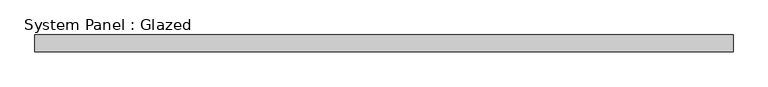
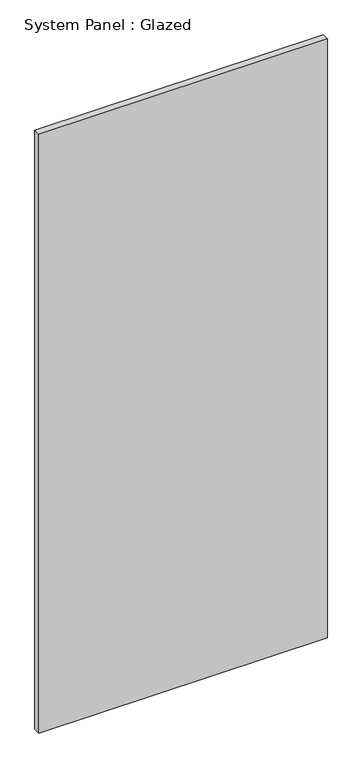
"""IFC4 building model written with IfcOpenShell, lengths in millimetres: plate geometry, System Panel : Glazed."""

from ifc_helpers import new_model, si_unit, origin, origin_with_axes, place, context, project, spatial, polyline, outline, extrude, source, transform, mapped, element, save


def system_panel_glazed_a93c8db9(model_context):
    return source(origin(), model_context, "Body", "SweptSolid", [
        extrude(outline(polyline([(527.05, 19.05), (-527.05, 19.05), (-527.05, 44.45), (527.05, 44.45), (527.05, 19.05)])), origin_with_axes(), (0.0, 0.0, 1.0), 2311.4),
    ])


if __name__ == "__main__":
    model = new_model("IFC4")
    model_context = context("Model", 3, world=origin())
    ifc_project = project(units=[si_unit("LENGTHUNIT", "METRE", prefix="MILLI")], contexts=[model_context])
    site = spatial("IfcSite", under=ifc_project)
    building = spatial("IfcBuilding", under=site)
    placement = place(None, origin())
    system_panel_glazed_shape = system_panel_glazed_a93c8db9(model_context)
    element("IfcPlate", 1, ObjectType="System Panel : Glazed", at=placement, inside=building, context=model_context, shape_type="MappedRepresentation", body=[
        mapped(system_panel_glazed_shape, transform((0.0, 0.0, 0.0), x_axis=(1.0, 0.0, 0.0), y_axis=(0.0, 1.0, 0.0), z_axis=(0.0, 0.0, 1.0))),
    ])
    save(model, "model.ifc")

# Revit data of these elements
# Type "System Panel : Glazed"
#   Construction Type Id = "GSP4R"
#   Analytic Construction = "1/8 in Pilkington single glazing"
#   Visual Light Transmittance = 0.9
#   Solar Heat Gain Coefficient = 0.86
#   Heat Transfer Coefficient (U) = 1.18115 BTU/(h·ft²·°F)
#   Define Thermal Properties by = 1
# Element 1 (IfcPlate, "System Panel : Glazed")
#   Materials on its faces: "Glass"
# Materials
#   "Glass": class "Glass", colour RGB 0 128 192, transparency 0.75, Description = "Soda Lime Glass", Cost = 0
